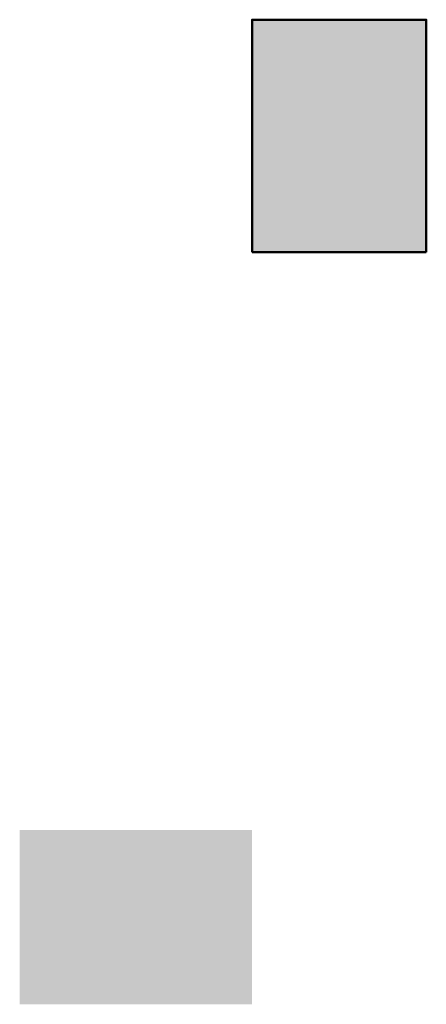
# Model space of a CAD drawing. Units: inches. Extents: x 2470 to 6338, y 1562 to 4199.
# Tile 5 of 5: x 6317 to 6338, y 4148 to 4199. Entities that reach past the tile are written whole.
import ezdxf

# ---------------------------------------------------------------- set-up
doc = ezdxf.new("R2010")
doc.units = ezdxf.units.IN
doc.layers.add('A-COLS', color=1, linetype='Continuous', lineweight=50)
doc.layers.add('A-COLS-PATT', color=1, linetype='Continuous', lineweight=18)

msp = doc.modelspace()

# ---------------------------------------------------------------- hatches: boundary and pattern name
at = {"layer": 'A-COLS-PATT'}
h = msp.add_hatch(color=256, dxfattribs=at)
h.dxf.hatch_style = 1
h.paths.add_polyline_path([(6338.049, 4198.772), (6329.049, 4198.772), (6329.049, 4189.772), (6329.049, 4186.772), (6338.049, 4186.772), (6338.049, 4189.772)])
h.paths.add_polyline_path([(6329.049, 4156.935), (6320.049, 4156.935), (6317.049, 4156.935), (6317.049, 4147.935), (6320.049, 4147.935), (6329.049, 4147.935)])

# ---------------------------------------------------------------- linework, layer by layer
at = {"layer": 'A-COLS'}
for p, q in [((6329.049, 4189.772), (6329.049, 4186.772)), ((6338.049, 4186.772), (6338.049, 4189.772)), ((6329.049, 4186.772), (6338.049, 4186.772))]:
    msp.add_line(p, q, dxfattribs=at)
msp.add_lwpolyline([(6329.049, 4189.772), (6329.049, 4198.772), (6338.049, 4198.772), (6338.049, 4189.772)], dxfattribs=at)

doc.saveas('drawing.dxf')
